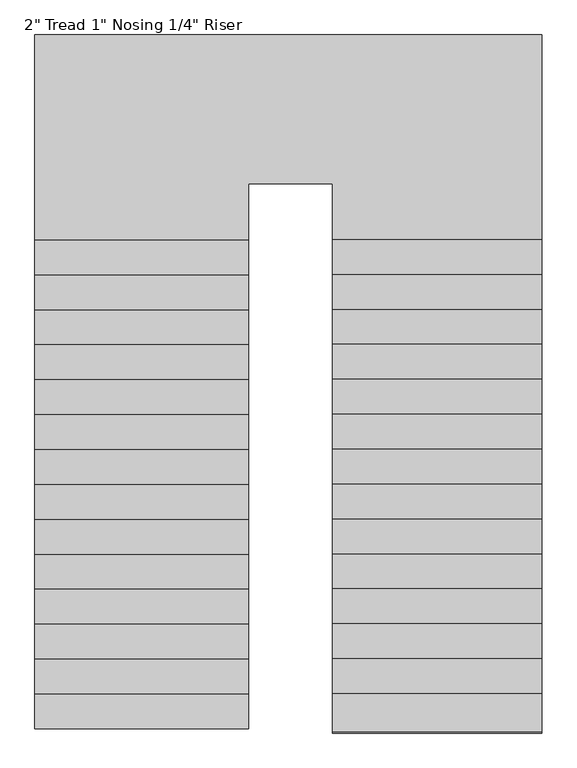
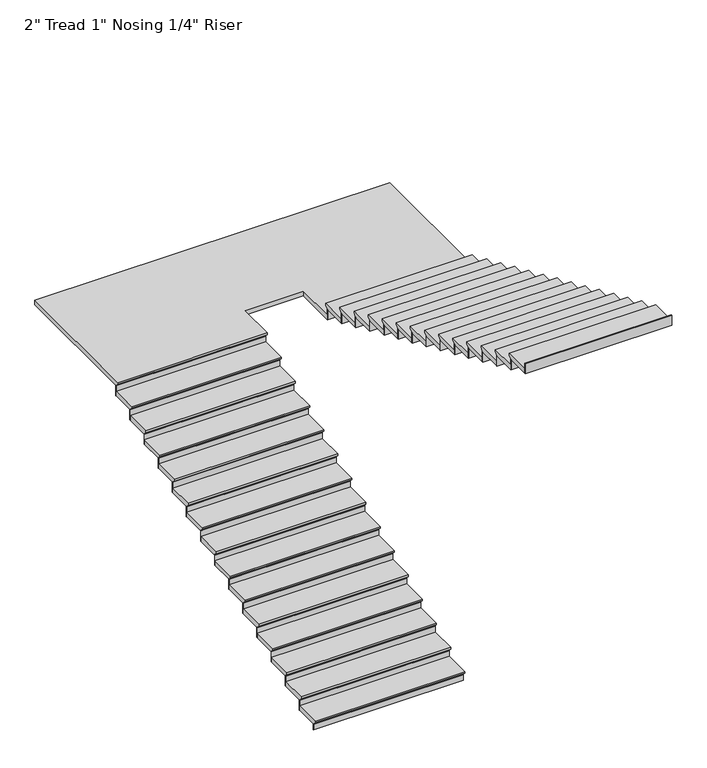
"""IFC4 building model written with IfcOpenShell, lengths in millimetres: stair flight geometry."""

from ifc_helpers import new_model, si_unit, origin, place, context, project, spatial, faceted_brep, source, transform, mapped, element, save


def stair_flight_303fa83b(model_context):
    return source(origin(), model_context, "Body", "Brep", [
        faceted_brep([(-5999.9290366, -6973.0610642, 11979.91), (-5999.9290366, -6973.0610642, 11998.96), (-7554.4415084, -6973.0610642, 11998.96), (-7554.4415084, -6973.0610642, 11979.91), (-5999.9290366, -6947.6610642, 11954.51), (-7554.4415084, -6947.6610642, 11954.51), (-5999.9290366, -6693.6610642, 11998.96), (-7554.4415084, -6693.6610642, 11998.96), (-7554.4415084, -6947.6610642, 11948.16), (-7554.4415084, -6693.6610642, 11948.16), (-5999.9290366, -6693.6610642, 11948.16), (-5999.9290366, -6947.6610642, 11948.16)], [[[0, 1, 2, 3]], [[4, 0, 3, 5]], [[2, 1, 6, 7]], [[8, 9, 10, 11]], [[2, 7, 9, 8, 5, 3]], [[8, 11, 4, 5]], [[6, 1, 0, 4, 11, 10]], [[7, 6, 10, 9]]]),
        faceted_brep([(-5999.9290366, -6947.6610642, 11948.16), (-5999.9290366, -6947.6610642, 11887.2), (-5999.9290366, -6941.3110642, 11887.2), (-5999.9290366, -6941.3110642, 11948.16), (-7554.4415084, -6947.6610642, 11948.16), (-7554.4415084, -6941.3110642, 11948.16), (-7554.4415084, -6941.3110642, 11887.2), (-7554.4415084, -6947.6610642, 11887.2)], [[[0, 1, 2, 3]], [[4, 5, 6, 7]], [[1, 0, 4, 7]], [[2, 1, 7, 6]], [[3, 2, 6, 5]], [[0, 3, 5, 4]]]),
        faceted_brep([(-5999.9290366, -6693.6610642, 12059.92), (-5999.9290366, -6693.6610642, 11948.16), (-5999.9290366, -6687.3110642, 11948.16), (-5999.9290366, -6687.3110642, 12059.92), (-7554.4415084, -6693.6610642, 12059.92), (-7554.4415084, -6687.3110642, 12059.92), (-7554.4415084, -6687.3110642, 11948.16), (-7554.4415084, -6693.6610642, 11948.16)], [[[0, 1, 2, 3]], [[4, 5, 6, 7]], [[1, 0, 4, 7]], [[2, 1, 7, 6]], [[3, 2, 6, 5]], [[0, 3, 5, 4]]]),
        faceted_brep([(-7554.4415084, -6719.0610642, 12110.72), (-5999.9290366, -6719.0610642, 12110.72), (-5999.9290366, -6439.6610642, 12110.72), (-7554.4415084, -6439.6610642, 12110.72), (-7554.4415084, -6693.6610642, 12059.92), (-7554.4415084, -6439.6610642, 12059.92), (-5999.9290366, -6439.6610642, 12059.92), (-5999.9290366, -6693.6610642, 12059.92), (-7554.4415084, -6693.6610642, 12066.27), (-7554.4415084, -6719.0610642, 12091.67), (-5999.9290366, -6693.6610642, 12066.27), (-5999.9290366, -6719.0610642, 12091.67)], [[[0, 1, 2, 3]], [[4, 5, 6, 7]], [[0, 3, 5, 4, 8, 9]], [[4, 7, 10, 8]], [[2, 1, 11, 10, 7, 6]], [[3, 2, 6, 5]], [[11, 1, 0, 9]], [[10, 11, 9, 8]]]),
        faceted_brep([(-5999.9290366, -6439.6610642, 12171.68), (-5999.9290366, -6439.6610642, 12059.92), (-5999.9290366, -6433.3110642, 12059.92), (-5999.9290366, -6433.3110642, 12171.68), (-7554.4415084, -6439.6610642, 12171.68), (-7554.4415084, -6433.3110642, 12171.68), (-7554.4415084, -6433.3110642, 12059.92), (-7554.4415084, -6439.6610642, 12059.92)], [[[0, 1, 2, 3]], [[4, 5, 6, 7]], [[1, 0, 4, 7]], [[2, 1, 7, 6]], [[3, 2, 6, 5]], [[0, 3, 5, 4]]]),
        faceted_brep([(-7554.4415084, -6465.0610642, 12222.48), (-5999.9290366, -6465.0610642, 12222.48), (-5999.9290366, -6185.6610642, 12222.48), (-7554.4415084, -6185.6610642, 12222.48), (-7554.4415084, -6439.6610642, 12171.68), (-7554.4415084, -6185.6610642, 12171.68), (-5999.9290366, -6185.6610642, 12171.68), (-5999.9290366, -6439.6610642, 12171.68), (-7554.4415084, -6439.6610642, 12178.03), (-7554.4415084, -6465.0610642, 12203.43), (-5999.9290366, -6439.6610642, 12178.03), (-5999.9290366, -6465.0610642, 12203.43)], [[[0, 1, 2, 3]], [[4, 5, 6, 7]], [[0, 3, 5, 4, 8, 9]], [[4, 7, 10, 8]], [[2, 1, 11, 10, 7, 6]], [[3, 2, 6, 5]], [[11, 1, 0, 9]], [[10, 11, 9, 8]]]),
        faceted_brep([(-5999.9290366, -6185.6610642, 12283.44), (-5999.9290366, -6185.6610642, 12171.68), (-5999.9290366, -6179.3110642, 12171.68), (-5999.9290366, -6179.3110642, 12283.44), (-7554.4415084, -6185.6610642, 12283.44), (-7554.4415084, -6179.3110642, 12283.44), (-7554.4415084, -6179.3110642, 12171.68), (-7554.4415084, -6185.6610642, 12171.68)], [[[0, 1, 2, 3]], [[4, 5, 6, 7]], [[1, 0, 4, 7]], [[2, 1, 7, 6]], [[3, 2, 6, 5]], [[0, 3, 5, 4]]]),
        faceted_brep([(-7554.4415084, -6211.0610642, 12334.24), (-5999.9290366, -6211.0610642, 12334.24), (-5999.9290366, -5931.6610642, 12334.24), (-7554.4415084, -5931.6610642, 12334.24), (-7554.4415084, -6185.6610642, 12283.44), (-7554.4415084, -5931.6610642, 12283.44), (-5999.9290366, -5931.6610642, 12283.44), (-5999.9290366, -6185.6610642, 12283.44), (-7554.4415084, -6185.6610642, 12289.79), (-7554.4415084, -6211.0610642, 12315.19), (-5999.9290366, -6185.6610642, 12289.79), (-5999.9290366, -6211.0610642, 12315.19)], [[[0, 1, 2, 3]], [[4, 5, 6, 7]], [[0, 3, 5, 4, 8, 9]], [[4, 7, 10, 8]], [[2, 1, 11, 10, 7, 6]], [[3, 2, 6, 5]], [[11, 1, 0, 9]], [[10, 11, 9, 8]]]),
        faceted_brep([(-5999.9290366, -5931.6610642, 12395.2), (-5999.9290366, -5931.6610642, 12283.44), (-5999.9290366, -5925.3110642, 12283.44), (-5999.9290366, -5925.3110642, 12395.2), (-7554.4415084, -5931.6610642, 12395.2), (-7554.4415084, -5925.3110642, 12395.2), (-7554.4415084, -5925.3110642, 12283.44), (-7554.4415084, -5931.6610642, 12283.44)], [[[0, 1, 2, 3]], [[4, 5, 6, 7]], [[1, 0, 4, 7]], [[2, 1, 7, 6]], [[3, 2, 6, 5]], [[0, 3, 5, 4]]]),
        faceted_brep([(-7554.4415084, -5957.0610642, 12446.0), (-5999.9290366, -5957.0610642, 12446.0), (-5999.9290366, -5677.6610642, 12446.0), (-7554.4415084, -5677.6610642, 12446.0), (-7554.4415084, -5931.6610642, 12395.2), (-7554.4415084, -5677.6610642, 12395.2), (-5999.9290366, -5677.6610642, 12395.2), (-5999.9290366, -5931.6610642, 12395.2), (-7554.4415084, -5931.6610642, 12401.55), (-7554.4415084, -5957.0610642, 12426.95), (-5999.9290366, -5931.6610642, 12401.55), (-5999.9290366, -5957.0610642, 12426.95)], [[[0, 1, 2, 3]], [[4, 5, 6, 7]], [[0, 3, 5, 4, 8, 9]], [[4, 7, 10, 8]], [[2, 1, 11, 10, 7, 6]], [[3, 2, 6, 5]], [[11, 1, 0, 9]], [[10, 11, 9, 8]]]),
        faceted_brep([(-5999.9290366, -5677.6610642, 12506.96), (-5999.9290366, -5677.6610642, 12395.2), (-5999.9290366, -5671.3110642, 12395.2), (-5999.9290366, -5671.3110642, 12506.96), (-7554.4415084, -5677.6610642, 12506.96), (-7554.4415084, -5671.3110642, 12506.96), (-7554.4415084, -5671.3110642, 12395.2), (-7554.4415084, -5677.6610642, 12395.2)], [[[0, 1, 2, 3]], [[4, 5, 6, 7]], [[1, 0, 4, 7]], [[2, 1, 7, 6]], [[3, 2, 6, 5]], [[0, 3, 5, 4]]]),
        faceted_brep([(-7554.4415084, -5703.0610642, 12557.76), (-5999.9290366, -5703.0610642, 12557.76), (-5999.9290366, -5423.6610642, 12557.76), (-7554.4415084, -5423.6610642, 12557.76), (-7554.4415084, -5677.6610642, 12506.96), (-7554.4415084, -5423.6610642, 12506.96), (-5999.9290366, -5423.6610642, 12506.96), (-5999.9290366, -5677.6610642, 12506.96), (-7554.4415084, -5677.6610642, 12513.31), (-7554.4415084, -5703.0610642, 12538.71), (-5999.9290366, -5677.6610642, 12513.31), (-5999.9290366, -5703.0610642, 12538.71)], [[[0, 1, 2, 3]], [[4, 5, 6, 7]], [[0, 3, 5, 4, 8, 9]], [[4, 7, 10, 8]], [[2, 1, 11, 10, 7, 6]], [[3, 2, 6, 5]], [[11, 1, 0, 9]], [[10, 11, 9, 8]]]),
        faceted_brep([(-5999.9290366, -5423.6610642, 12618.72), (-5999.9290366, -5423.6610642, 12506.96), (-5999.9290366, -5417.3110642, 12506.96), (-5999.9290366, -5417.3110642, 12618.72), (-7554.4415084, -5423.6610642, 12618.72), (-7554.4415084, -5417.3110642, 12618.72), (-7554.4415084, -5417.3110642, 12506.96), (-7554.4415084, -5423.6610642, 12506.96)], [[[0, 1, 2, 3]], [[4, 5, 6, 7]], [[1, 0, 4, 7]], [[2, 1, 7, 6]], [[3, 2, 6, 5]], [[0, 3, 5, 4]]]),
        faceted_brep([(-7554.4415084, -5449.0610642, 12669.52), (-5999.9290366, -5449.0610642, 12669.52), (-5999.9290366, -5169.6610642, 12669.52), (-7554.4415084, -5169.6610642, 12669.52), (-7554.4415084, -5423.6610642, 12618.72), (-7554.4415084, -5169.6610642, 12618.72), (-5999.9290366, -5169.6610642, 12618.72), (-5999.9290366, -5423.6610642, 12618.72), (-7554.4415084, -5423.6610642, 12625.07), (-7554.4415084, -5449.0610642, 12650.47), (-5999.9290366, -5423.6610642, 12625.07), (-5999.9290366, -5449.0610642, 12650.47)], [[[0, 1, 2, 3]], [[4, 5, 6, 7]], [[0, 3, 5, 4, 8, 9]], [[4, 7, 10, 8]], [[2, 1, 11, 10, 7, 6]], [[3, 2, 6, 5]], [[11, 1, 0, 9]], [[10, 11, 9, 8]]]),
        faceted_brep([(-5999.9290366, -5169.6610642, 12730.48), (-5999.9290366, -5169.6610642, 12618.72), (-5999.9290366, -5163.3110642, 12618.72), (-5999.9290366, -5163.3110642, 12730.48), (-7554.4415084, -5169.6610642, 12730.48), (-7554.4415084, -5163.3110642, 12730.48), (-7554.4415084, -5163.3110642, 12618.72), (-7554.4415084, -5169.6610642, 12618.72)], [[[0, 1, 2, 3]], [[4, 5, 6, 7]], [[1, 0, 4, 7]], [[2, 1, 7, 6]], [[3, 2, 6, 5]], [[0, 3, 5, 4]]]),
        faceted_brep([(-7554.4415084, -5195.0610642, 12781.28), (-5999.9290366, -5195.0610642, 12781.28), (-5999.9290366, -4915.6610642, 12781.28), (-7554.4415084, -4915.6610642, 12781.28), (-7554.4415084, -5169.6610642, 12730.48), (-7554.4415084, -4915.6610642, 12730.48), (-5999.9290366, -4915.6610642, 12730.48), (-5999.9290366, -5169.6610642, 12730.48), (-7554.4415084, -5169.6610642, 12736.83), (-7554.4415084, -5195.0610642, 12762.23), (-5999.9290366, -5169.6610642, 12736.83), (-5999.9290366, -5195.0610642, 12762.23)], [[[0, 1, 2, 3]], [[4, 5, 6, 7]], [[0, 3, 5, 4, 8, 9]], [[4, 7, 10, 8]], [[2, 1, 11, 10, 7, 6]], [[3, 2, 6, 5]], [[11, 1, 0, 9]], [[10, 11, 9, 8]]]),
        faceted_brep([(-5999.9290366, -4915.6610642, 12842.24), (-5999.9290366, -4915.6610642, 12730.48), (-5999.9290366, -4909.3110642, 12730.48), (-5999.9290366, -4909.3110642, 12842.24), (-7554.4415084, -4915.6610642, 12842.24), (-7554.4415084, -4909.3110642, 12842.24), (-7554.4415084, -4909.3110642, 12730.48), (-7554.4415084, -4915.6610642, 12730.48)], [[[0, 1, 2, 3]], [[4, 5, 6, 7]], [[1, 0, 4, 7]], [[2, 1, 7, 6]], [[3, 2, 6, 5]], [[0, 3, 5, 4]]]),
        faceted_brep([(-7554.4415084, -4941.0610642, 12893.04), (-5999.9290366, -4941.0610642, 12893.04), (-5999.9290366, -4661.6610642, 12893.04), (-7554.4415084, -4661.6610642, 12893.04), (-7554.4415084, -4915.6610642, 12842.24), (-7554.4415084, -4661.6610642, 12842.24), (-5999.9290366, -4661.6610642, 12842.24), (-5999.9290366, -4915.6610642, 12842.24), (-7554.4415084, -4915.6610642, 12848.59), (-7554.4415084, -4941.0610642, 12873.99), (-5999.9290366, -4915.6610642, 12848.59), (-5999.9290366, -4941.0610642, 12873.99)], [[[0, 1, 2, 3]], [[4, 5, 6, 7]], [[0, 3, 5, 4, 8, 9]], [[4, 7, 10, 8]], [[2, 1, 11, 10, 7, 6]], [[3, 2, 6, 5]], [[11, 1, 0, 9]], [[10, 11, 9, 8]]]),
        faceted_brep([(-5999.9290366, -4661.6610642, 12954.0), (-5999.9290366, -4661.6610642, 12842.24), (-5999.9290366, -4655.3110642, 12842.24), (-5999.9290366, -4655.3110642, 12954.0), (-7554.4415084, -4661.6610642, 12954.0), (-7554.4415084, -4655.3110642, 12954.0), (-7554.4415084, -4655.3110642, 12842.24), (-7554.4415084, -4661.6610642, 12842.24)], [[[0, 1, 2, 3]], [[4, 5, 6, 7]], [[1, 0, 4, 7]], [[2, 1, 7, 6]], [[3, 2, 6, 5]], [[0, 3, 5, 4]]]),
        faceted_brep([(-7554.4415084, -4687.0610642, 13004.8), (-5999.9290366, -4687.0610642, 13004.8), (-5999.9290366, -4407.6610642, 13004.8), (-7554.4415084, -4407.6610642, 13004.8), (-7554.4415084, -4661.6610642, 12954.0), (-7554.4415084, -4407.6610642, 12954.0), (-5999.9290366, -4407.6610642, 12954.0), (-5999.9290366, -4661.6610642, 12954.0), (-7554.4415084, -4661.6610642, 12960.35), (-7554.4415084, -4687.0610642, 12985.75), (-5999.9290366, -4661.6610642, 12960.35), (-5999.9290366, -4687.0610642, 12985.75)], [[[0, 1, 2, 3]], [[4, 5, 6, 7]], [[0, 3, 5, 4, 8, 9]], [[4, 7, 10, 8]], [[2, 1, 11, 10, 7, 6]], [[3, 2, 6, 5]], [[11, 1, 0, 9]], [[10, 11, 9, 8]]]),
        faceted_brep([(-5999.9290366, -4407.6610642, 13065.76), (-5999.9290366, -4407.6610642, 12954.0), (-5999.9290366, -4401.3110642, 12954.0), (-5999.9290366, -4401.3110642, 13065.76), (-7554.4415084, -4407.6610642, 13065.76), (-7554.4415084, -4401.3110642, 13065.76), (-7554.4415084, -4401.3110642, 12954.0), (-7554.4415084, -4407.6610642, 12954.0)], [[[0, 1, 2, 3]], [[4, 5, 6, 7]], [[1, 0, 4, 7]], [[2, 1, 7, 6]], [[3, 2, 6, 5]], [[0, 3, 5, 4]]]),
        faceted_brep([(-7554.4415084, -4433.0610642, 13116.56), (-5999.9290366, -4433.0610642, 13116.56), (-5999.9290366, -4153.6610642, 13116.56), (-7554.4415084, -4153.6610642, 13116.56), (-7554.4415084, -4407.6610642, 13065.76), (-7554.4415084, -4153.6610642, 13065.76), (-5999.9290366, -4153.6610642, 13065.76), (-5999.9290366, -4407.6610642, 13065.76), (-7554.4415084, -4407.6610642, 13072.11), (-7554.4415084, -4433.0610642, 13097.51), (-5999.9290366, -4407.6610642, 13072.11), (-5999.9290366, -4433.0610642, 13097.51)], [[[0, 1, 2, 3]], [[4, 5, 6, 7]], [[0, 3, 5, 4, 8, 9]], [[4, 7, 10, 8]], [[2, 1, 11, 10, 7, 6]], [[3, 2, 6, 5]], [[11, 1, 0, 9]], [[10, 11, 9, 8]]]),
        faceted_brep([(-5999.9290366, -4153.6610642, 13177.52), (-5999.9290366, -4153.6610642, 13065.76), (-5999.9290366, -4147.3110642, 13065.76), (-5999.9290366, -4147.3110642, 13177.52), (-7554.4415084, -4153.6610642, 13177.52), (-7554.4415084, -4147.3110642, 13177.52), (-7554.4415084, -4147.3110642, 13065.76), (-7554.4415084, -4153.6610642, 13065.76)], [[[0, 1, 2, 3]], [[4, 5, 6, 7]], [[1, 0, 4, 7]], [[2, 1, 7, 6]], [[3, 2, 6, 5]], [[0, 3, 5, 4]]]),
        faceted_brep([(-7554.4415084, -4179.0610642, 13228.32), (-5999.9290366, -4179.0610642, 13228.32), (-5999.9290366, -3899.6610642, 13228.32), (-7554.4415084, -3899.6610642, 13228.32), (-7554.4415084, -4153.6610642, 13177.52), (-7554.4415084, -3899.6610642, 13177.52), (-5999.9290366, -3899.6610642, 13177.52), (-5999.9290366, -4153.6610642, 13177.52), (-7554.4415084, -4153.6610642, 13183.87), (-7554.4415084, -4179.0610642, 13209.27), (-5999.9290366, -4153.6610642, 13183.87), (-5999.9290366, -4179.0610642, 13209.27)], [[[0, 1, 2, 3]], [[4, 5, 6, 7]], [[0, 3, 5, 4, 8, 9]], [[4, 7, 10, 8]], [[2, 1, 11, 10, 7, 6]], [[3, 2, 6, 5]], [[11, 1, 0, 9]], [[10, 11, 9, 8]]]),
        faceted_brep([(-5999.9290366, -3899.6610642, 13289.28), (-5999.9290366, -3899.6610642, 13177.52), (-5999.9290366, -3893.3110642, 13177.52), (-5999.9290366, -3893.3110642, 13289.28), (-7554.4415084, -3899.6610642, 13289.28), (-7554.4415084, -3893.3110642, 13289.28), (-7554.4415084, -3893.3110642, 13177.52), (-7554.4415084, -3899.6610642, 13177.52)], [[[0, 1, 2, 3]], [[4, 5, 6, 7]], [[1, 0, 4, 7]], [[2, 1, 7, 6]], [[3, 2, 6, 5]], [[0, 3, 5, 4]]]),
        faceted_brep([(-7554.4415084, -3925.0610642, 13340.08), (-5999.9290366, -3925.0610642, 13340.08), (-5999.9290366, -3645.6610642, 13340.08), (-7554.4415084, -3645.6610642, 13340.08), (-7554.4415084, -3899.6610642, 13289.28), (-7554.4415084, -3645.6610642, 13289.28), (-5999.9290366, -3645.6610642, 13289.28), (-5999.9290366, -3899.6610642, 13289.28), (-7554.4415084, -3899.6610642, 13295.63), (-7554.4415084, -3925.0610642, 13321.03), (-5999.9290366, -3899.6610642, 13295.63), (-5999.9290366, -3925.0610642, 13321.03)], [[[0, 1, 2, 3]], [[4, 5, 6, 7]], [[0, 3, 5, 4, 8, 9]], [[4, 7, 10, 8]], [[2, 1, 11, 10, 7, 6]], [[3, 2, 6, 5]], [[11, 1, 0, 9]], [[10, 11, 9, 8]]]),
        faceted_brep([(-5999.9290366, -3645.6610642, 13401.04), (-5999.9290366, -3645.6610642, 13289.28), (-5999.9290366, -3639.3110642, 13289.28), (-5999.9290366, -3639.3110642, 13401.04), (-7554.4415084, -3645.6610642, 13401.04), (-7554.4415084, -3639.3110642, 13401.04), (-7554.4415084, -3639.3110642, 13289.28), (-7554.4415084, -3645.6610642, 13289.28)], [[[0, 1, 2, 3]], [[4, 5, 6, 7]], [[1, 0, 4, 7]], [[2, 1, 7, 6]], [[3, 2, 6, 5]], [[0, 3, 5, 4]]]),
        faceted_brep([(-7554.4415084, -3671.0610642, 13451.84), (-5999.9290366, -3671.0610642, 13451.84), (-5999.9290366, -3391.6610642, 13451.84), (-7554.4415084, -3391.6610642, 13451.84), (-7554.4415084, -3645.6610642, 13401.04), (-7554.4415084, -3391.6610642, 13401.04), (-5999.9290366, -3391.6610642, 13401.04), (-5999.9290366, -3645.6610642, 13401.04), (-7554.4415084, -3645.6610642, 13407.39), (-7554.4415084, -3671.0610642, 13432.79), (-5999.9290366, -3645.6610642, 13407.39), (-5999.9290366, -3671.0610642, 13432.79)], [[[0, 1, 2, 3]], [[4, 5, 6, 7]], [[0, 3, 5, 4, 8, 9]], [[4, 7, 10, 8]], [[2, 1, 11, 10, 7, 6]], [[3, 2, 6, 5]], [[11, 1, 0, 9]], [[10, 11, 9, 8]]]),
        faceted_brep([(-5999.9290366, -3391.6610642, 13512.8), (-5999.9290366, -3391.6610642, 13401.04), (-5999.9290366, -3385.3110642, 13401.04), (-5999.9290366, -3385.3110642, 13512.8), (-7554.4415084, -3391.6610642, 13512.8), (-7554.4415084, -3385.3110642, 13512.8), (-7554.4415084, -3385.3110642, 13401.04), (-7554.4415084, -3391.6610642, 13401.04)], [[[0, 1, 2, 3]], [[4, 5, 6, 7]], [[1, 0, 4, 7]], [[2, 1, 7, 6]], [[3, 2, 6, 5]], [[0, 3, 5, 4]]]),
        faceted_brep([(-3866.3290366, -3442.4610642, 13563.6), (-3866.3290366, -1928.4217109, 13563.6), (-7554.4415084, -1928.4217109, 13563.6), (-7554.4415084, -3417.0610642, 13563.6), (-5999.9290366, -3417.0610642, 13563.6), (-5999.9290366, -3010.6610642, 13563.6), (-5390.3290366, -3010.6610642, 13563.6), (-5390.3290366, -3442.4610642, 13563.6), (-3866.3290366, -1928.4217109, 13512.8), (-3866.3290366, -3442.4610642, 13512.8), (-5390.3290366, -3442.4610642, 13512.8), (-5390.3290366, -3010.6610642, 13512.8), (-5999.9290366, -3010.6610642, 13512.8), (-5999.9290366, -3391.6610642, 13512.8), (-7554.4415084, -3391.6610642, 13512.8), (-7554.4415084, -1928.4217109, 13512.8), (-7554.4415084, -3391.6610642, 13519.15), (-7554.4415084, -3417.0610642, 13544.55), (-5999.9290366, -3391.6610642, 13519.15), (-5999.9290366, -3417.0610642, 13544.55)], [[[0, 1, 2, 3, 4, 5, 6, 7]], [[8, 9, 10, 11, 12, 13, 14, 15]], [[1, 0, 9, 8]], [[2, 1, 8, 15]], [[3, 2, 15, 14, 16, 17]], [[14, 13, 18, 16]], [[5, 4, 19, 18, 13, 12]], [[6, 5, 12, 11]], [[7, 6, 11, 10]], [[0, 7, 10, 9]], [[19, 4, 3, 17]], [[18, 19, 17, 16]]]),
        faceted_brep([(-5390.3290366, -3442.4610642, 13624.56), (-5390.3290366, -3442.4610642, 13512.8), (-5390.3290366, -3448.8110642, 13512.8), (-5390.3290366, -3448.8110642, 13624.56), (-3866.3290366, -3442.4610642, 13624.56), (-3866.3290366, -3448.8110642, 13624.56), (-3866.3290366, -3448.8110642, 13512.8), (-3866.3290366, -3442.4610642, 13512.8)], [[[0, 1, 2, 3]], [[4, 5, 6, 7]], [[1, 0, 4, 7]], [[2, 1, 7, 6]], [[3, 2, 6, 5]], [[0, 3, 5, 4]]]),
        faceted_brep([(-3866.3290366, -3417.0610642, 13675.36), (-5390.3290366, -3417.0610642, 13675.36), (-5390.3290366, -3696.4610642, 13675.36), (-3866.3290366, -3696.4610642, 13675.36), (-3866.3290366, -3442.4610642, 13624.56), (-3866.3290366, -3696.4610642, 13624.56), (-5390.3290366, -3696.4610642, 13624.56), (-5390.3290366, -3442.4610642, 13624.56), (-3866.3290366, -3442.4610642, 13630.91), (-3866.3290366, -3417.0610642, 13656.31), (-5390.3290366, -3442.4610642, 13630.91), (-5390.3290366, -3417.0610642, 13656.31)], [[[0, 1, 2, 3]], [[4, 5, 6, 7]], [[0, 3, 5, 4, 8, 9]], [[4, 7, 10, 8]], [[2, 1, 11, 10, 7, 6]], [[3, 2, 6, 5]], [[11, 1, 0, 9]], [[10, 11, 9, 8]]]),
        faceted_brep([(-5390.3290366, -3696.4610642, 13736.32), (-5390.3290366, -3696.4610642, 13624.56), (-5390.3290366, -3702.8110642, 13624.56), (-5390.3290366, -3702.8110642, 13736.32), (-3866.3290366, -3696.4610642, 13736.32), (-3866.3290366, -3702.8110642, 13736.32), (-3866.3290366, -3702.8110642, 13624.56), (-3866.3290366, -3696.4610642, 13624.56)], [[[0, 1, 2, 3]], [[4, 5, 6, 7]], [[1, 0, 4, 7]], [[2, 1, 7, 6]], [[3, 2, 6, 5]], [[0, 3, 5, 4]]]),
        faceted_brep([(-3866.3290366, -3671.0610642, 13787.12), (-5390.3290366, -3671.0610642, 13787.12), (-5390.3290366, -3950.4610642, 13787.12), (-3866.3290366, -3950.4610642, 13787.12), (-3866.3290366, -3696.4610642, 13736.32), (-3866.3290366, -3950.4610642, 13736.32), (-5390.3290366, -3950.4610642, 13736.32), (-5390.3290366, -3696.4610642, 13736.32), (-3866.3290366, -3696.4610642, 13742.67), (-3866.3290366, -3671.0610642, 13768.07), (-5390.3290366, -3696.4610642, 13742.67), (-5390.3290366, -3671.0610642, 13768.07)], [[[0, 1, 2, 3]], [[4, 5, 6, 7]], [[0, 3, 5, 4, 8, 9]], [[4, 7, 10, 8]], [[2, 1, 11, 10, 7, 6]], [[3, 2, 6, 5]], [[11, 1, 0, 9]], [[10, 11, 9, 8]]]),
        faceted_brep([(-5390.3290366, -3950.4610642, 13848.08), (-5390.3290366, -3950.4610642, 13736.32), (-5390.3290366, -3956.8110642, 13736.32), (-5390.3290366, -3956.8110642, 13848.08), (-3866.3290366, -3950.4610642, 13848.08), (-3866.3290366, -3956.8110642, 13848.08), (-3866.3290366, -3956.8110642, 13736.32), (-3866.3290366, -3950.4610642, 13736.32)], [[[0, 1, 2, 3]], [[4, 5, 6, 7]], [[1, 0, 4, 7]], [[2, 1, 7, 6]], [[3, 2, 6, 5]], [[0, 3, 5, 4]]]),
        faceted_brep([(-3866.3290366, -3925.0610642, 13898.88), (-5390.3290366, -3925.0610642, 13898.88), (-5390.3290366, -4204.4610642, 13898.88), (-3866.3290366, -4204.4610642, 13898.88), (-3866.3290366, -3950.4610642, 13848.08), (-3866.3290366, -4204.4610642, 13848.08), (-5390.3290366, -4204.4610642, 13848.08), (-5390.3290366, -3950.4610642, 13848.08), (-3866.3290366, -3950.4610642, 13854.43), (-3866.3290366, -3925.0610642, 13879.83), (-5390.3290366, -3950.4610642, 13854.43), (-5390.3290366, -3925.0610642, 13879.83)], [[[0, 1, 2, 3]], [[4, 5, 6, 7]], [[0, 3, 5, 4, 8, 9]], [[4, 7, 10, 8]], [[2, 1, 11, 10, 7, 6]], [[3, 2, 6, 5]], [[11, 1, 0, 9]], [[10, 11, 9, 8]]]),
        faceted_brep([(-5390.3290366, -4204.4610642, 13959.84), (-5390.3290366, -4204.4610642, 13848.08), (-5390.3290366, -4210.8110642, 13848.08), (-5390.3290366, -4210.8110642, 13959.84), (-3866.3290366, -4204.4610642, 13959.84), (-3866.3290366, -4210.8110642, 13959.84), (-3866.3290366, -4210.8110642, 13848.08), (-3866.3290366, -4204.4610642, 13848.08)], [[[0, 1, 2, 3]], [[4, 5, 6, 7]], [[1, 0, 4, 7]], [[2, 1, 7, 6]], [[3, 2, 6, 5]], [[0, 3, 5, 4]]]),
        faceted_brep([(-3866.3290366, -4179.0610642, 14010.64), (-5390.3290366, -4179.0610642, 14010.64), (-5390.3290366, -4458.4610642, 14010.64), (-3866.3290366, -4458.4610642, 14010.64), (-3866.3290366, -4204.4610642, 13959.84), (-3866.3290366, -4458.4610642, 13959.84), (-5390.3290366, -4458.4610642, 13959.84), (-5390.3290366, -4204.4610642, 13959.84), (-3866.3290366, -4204.4610642, 13966.19), (-3866.3290366, -4179.0610642, 13991.59), (-5390.3290366, -4204.4610642, 13966.19), (-5390.3290366, -4179.0610642, 13991.59)], [[[0, 1, 2, 3]], [[4, 5, 6, 7]], [[0, 3, 5, 4, 8, 9]], [[4, 7, 10, 8]], [[2, 1, 11, 10, 7, 6]], [[3, 2, 6, 5]], [[11, 1, 0, 9]], [[10, 11, 9, 8]]]),
        faceted_brep([(-5390.3290366, -4458.4610642, 14071.6), (-5390.3290366, -4458.4610642, 13959.84), (-5390.3290366, -4464.8110642, 13959.84), (-5390.3290366, -4464.8110642, 14071.6), (-3866.3290366, -4458.4610642, 14071.6), (-3866.3290366, -4464.8110642, 14071.6), (-3866.3290366, -4464.8110642, 13959.84), (-3866.3290366, -4458.4610642, 13959.84)], [[[0, 1, 2, 3]], [[4, 5, 6, 7]], [[1, 0, 4, 7]], [[2, 1, 7, 6]], [[3, 2, 6, 5]], [[0, 3, 5, 4]]]),
        faceted_brep([(-3866.3290366, -4433.0610642, 14122.4), (-5390.3290366, -4433.0610642, 14122.4), (-5390.3290366, -4712.4610642, 14122.4), (-3866.3290366, -4712.4610642, 14122.4), (-3866.3290366, -4458.4610642, 14071.6), (-3866.3290366, -4712.4610642, 14071.6), (-5390.3290366, -4712.4610642, 14071.6), (-5390.3290366, -4458.4610642, 14071.6), (-3866.3290366, -4458.4610642, 14077.95), (-3866.3290366, -4433.0610642, 14103.35), (-5390.3290366, -4458.4610642, 14077.95), (-5390.3290366, -4433.0610642, 14103.35)], [[[0, 1, 2, 3]], [[4, 5, 6, 7]], [[0, 3, 5, 4, 8, 9]], [[4, 7, 10, 8]], [[2, 1, 11, 10, 7, 6]], [[3, 2, 6, 5]], [[11, 1, 0, 9]], [[10, 11, 9, 8]]]),
        faceted_brep([(-5390.3290366, -4712.4610642, 14183.36), (-5390.3290366, -4712.4610642, 14071.6), (-5390.3290366, -4718.8110642, 14071.6), (-5390.3290366, -4718.8110642, 14183.36), (-3866.3290366, -4712.4610642, 14183.36), (-3866.3290366, -4718.8110642, 14183.36), (-3866.3290366, -4718.8110642, 14071.6), (-3866.3290366, -4712.4610642, 14071.6)], [[[0, 1, 2, 3]], [[4, 5, 6, 7]], [[1, 0, 4, 7]], [[2, 1, 7, 6]], [[3, 2, 6, 5]], [[0, 3, 5, 4]]]),
        faceted_brep([(-3866.3290366, -4687.0610642, 14234.16), (-5390.3290366, -4687.0610642, 14234.16), (-5390.3290366, -4966.4610642, 14234.16), (-3866.3290366, -4966.4610642, 14234.16), (-3866.3290366, -4712.4610642, 14183.36), (-3866.3290366, -4966.4610642, 14183.36), (-5390.3290366, -4966.4610642, 14183.36), (-5390.3290366, -4712.4610642, 14183.36), (-3866.3290366, -4712.4610642, 14189.71), (-3866.3290366, -4687.0610642, 14215.11), (-5390.3290366, -4712.4610642, 14189.71), (-5390.3290366, -4687.0610642, 14215.11)], [[[0, 1, 2, 3]], [[4, 5, 6, 7]], [[0, 3, 5, 4, 8, 9]], [[4, 7, 10, 8]], [[2, 1, 11, 10, 7, 6]], [[3, 2, 6, 5]], [[11, 1, 0, 9]], [[10, 11, 9, 8]]]),
        faceted_brep([(-5390.3290366, -4966.4610642, 14295.12), (-5390.3290366, -4966.4610642, 14183.36), (-5390.3290366, -4972.8110642, 14183.36), (-5390.3290366, -4972.8110642, 14295.12), (-3866.3290366, -4966.4610642, 14295.12), (-3866.3290366, -4972.8110642, 14295.12), (-3866.3290366, -4972.8110642, 14183.36), (-3866.3290366, -4966.4610642, 14183.36)], [[[0, 1, 2, 3]], [[4, 5, 6, 7]], [[1, 0, 4, 7]], [[2, 1, 7, 6]], [[3, 2, 6, 5]], [[0, 3, 5, 4]]]),
        faceted_brep([(-3866.3290366, -4941.0610642, 14345.92), (-5390.3290366, -4941.0610642, 14345.92), (-5390.3290366, -5220.4610642, 14345.92), (-3866.3290366, -5220.4610642, 14345.92), (-3866.3290366, -4966.4610642, 14295.12), (-3866.3290366, -5220.4610642, 14295.12), (-5390.3290366, -5220.4610642, 14295.12), (-5390.3290366, -4966.4610642, 14295.12), (-3866.3290366, -4966.4610642, 14301.47), (-3866.3290366, -4941.0610642, 14326.87), (-5390.3290366, -4966.4610642, 14301.47), (-5390.3290366, -4941.0610642, 14326.87)], [[[0, 1, 2, 3]], [[4, 5, 6, 7]], [[0, 3, 5, 4, 8, 9]], [[4, 7, 10, 8]], [[2, 1, 11, 10, 7, 6]], [[3, 2, 6, 5]], [[11, 1, 0, 9]], [[10, 11, 9, 8]]]),
        faceted_brep([(-5390.3290366, -5220.4610642, 14406.88), (-5390.3290366, -5220.4610642, 14295.12), (-5390.3290366, -5226.8110642, 14295.12), (-5390.3290366, -5226.8110642, 14406.88), (-3866.3290366, -5220.4610642, 14406.88), (-3866.3290366, -5226.8110642, 14406.88), (-3866.3290366, -5226.8110642, 14295.12), (-3866.3290366, -5220.4610642, 14295.12)], [[[0, 1, 2, 3]], [[4, 5, 6, 7]], [[1, 0, 4, 7]], [[2, 1, 7, 6]], [[3, 2, 6, 5]], [[0, 3, 5, 4]]]),
        faceted_brep([(-3866.3290366, -5195.0610642, 14457.68), (-5390.3290366, -5195.0610642, 14457.68), (-5390.3290366, -5474.4610642, 14457.68), (-3866.3290366, -5474.4610642, 14457.68), (-3866.3290366, -5220.4610642, 14406.88), (-3866.3290366, -5474.4610642, 14406.88), (-5390.3290366, -5474.4610642, 14406.88), (-5390.3290366, -5220.4610642, 14406.88), (-3866.3290366, -5220.4610642, 14413.23), (-3866.3290366, -5195.0610642, 14438.63), (-5390.3290366, -5220.4610642, 14413.23), (-5390.3290366, -5195.0610642, 14438.63)], [[[0, 1, 2, 3]], [[4, 5, 6, 7]], [[0, 3, 5, 4, 8, 9]], [[4, 7, 10, 8]], [[2, 1, 11, 10, 7, 6]], [[3, 2, 6, 5]], [[11, 1, 0, 9]], [[10, 11, 9, 8]]]),
        faceted_brep([(-5390.3290366, -5474.4610642, 14518.64), (-5390.3290366, -5474.4610642, 14406.88), (-5390.3290366, -5480.8110642, 14406.88), (-5390.3290366, -5480.8110642, 14518.64), (-3866.3290366, -5474.4610642, 14518.64), (-3866.3290366, -5480.8110642, 14518.64), (-3866.3290366, -5480.8110642, 14406.88), (-3866.3290366, -5474.4610642, 14406.88)], [[[0, 1, 2, 3]], [[4, 5, 6, 7]], [[1, 0, 4, 7]], [[2, 1, 7, 6]], [[3, 2, 6, 5]], [[0, 3, 5, 4]]]),
        faceted_brep([(-3866.3290366, -5449.0610642, 14569.44), (-5390.3290366, -5449.0610642, 14569.44), (-5390.3290366, -5728.4610642, 14569.44), (-3866.3290366, -5728.4610642, 14569.44), (-3866.3290366, -5474.4610642, 14518.64), (-3866.3290366, -5728.4610642, 14518.64), (-5390.3290366, -5728.4610642, 14518.64), (-5390.3290366, -5474.4610642, 14518.64), (-3866.3290366, -5474.4610642, 14524.99), (-3866.3290366, -5449.0610642, 14550.39), (-5390.3290366, -5474.4610642, 14524.99), (-5390.3290366, -5449.0610642, 14550.39)], [[[0, 1, 2, 3]], [[4, 5, 6, 7]], [[0, 3, 5, 4, 8, 9]], [[4, 7, 10, 8]], [[2, 1, 11, 10, 7, 6]], [[3, 2, 6, 5]], [[11, 1, 0, 9]], [[10, 11, 9, 8]]]),
        faceted_brep([(-5390.3290366, -5728.4610642, 14630.4), (-5390.3290366, -5728.4610642, 14518.64), (-5390.3290366, -5734.8110642, 14518.64), (-5390.3290366, -5734.8110642, 14630.4), (-3866.3290366, -5728.4610642, 14630.4), (-3866.3290366, -5734.8110642, 14630.4), (-3866.3290366, -5734.8110642, 14518.64), (-3866.3290366, -5728.4610642, 14518.64)], [[[0, 1, 2, 3]], [[4, 5, 6, 7]], [[1, 0, 4, 7]], [[2, 1, 7, 6]], [[3, 2, 6, 5]], [[0, 3, 5, 4]]]),
        faceted_brep([(-3866.3290366, -5703.0610642, 14681.2), (-5390.3290366, -5703.0610642, 14681.2), (-5390.3290366, -5982.4610642, 14681.2), (-3866.3290366, -5982.4610642, 14681.2), (-3866.3290366, -5728.4610642, 14630.4), (-3866.3290366, -5982.4610642, 14630.4), (-5390.3290366, -5982.4610642, 14630.4), (-5390.3290366, -5728.4610642, 14630.4), (-3866.3290366, -5728.4610642, 14636.75), (-3866.3290366, -5703.0610642, 14662.15), (-5390.3290366, -5728.4610642, 14636.75), (-5390.3290366, -5703.0610642, 14662.15)], [[[0, 1, 2, 3]], [[4, 5, 6, 7]], [[0, 3, 5, 4, 8, 9]], [[4, 7, 10, 8]], [[2, 1, 11, 10, 7, 6]], [[3, 2, 6, 5]], [[11, 1, 0, 9]], [[10, 11, 9, 8]]]),
        faceted_brep([(-5390.3290366, -5982.4610642, 14742.16), (-5390.3290366, -5982.4610642, 14630.4), (-5390.3290366, -5988.8110642, 14630.4), (-5390.3290366, -5988.8110642, 14742.16), (-3866.3290366, -5982.4610642, 14742.16), (-3866.3290366, -5988.8110642, 14742.16), (-3866.3290366, -5988.8110642, 14630.4), (-3866.3290366, -5982.4610642, 14630.4)], [[[0, 1, 2, 3]], [[4, 5, 6, 7]], [[1, 0, 4, 7]], [[2, 1, 7, 6]], [[3, 2, 6, 5]], [[0, 3, 5, 4]]]),
        faceted_brep([(-3866.3290366, -5957.0610642, 14792.96), (-5390.3290366, -5957.0610642, 14792.96), (-5390.3290366, -6236.4610642, 14792.96), (-3866.3290366, -6236.4610642, 14792.96), (-3866.3290366, -5982.4610642, 14742.16), (-3866.3290366, -6236.4610642, 14742.16), (-5390.3290366, -6236.4610642, 14742.16), (-5390.3290366, -5982.4610642, 14742.16), (-3866.3290366, -5982.4610642, 14748.51), (-3866.3290366, -5957.0610642, 14773.91), (-5390.3290366, -5982.4610642, 14748.51), (-5390.3290366, -5957.0610642, 14773.91)], [[[0, 1, 2, 3]], [[4, 5, 6, 7]], [[0, 3, 5, 4, 8, 9]], [[4, 7, 10, 8]], [[2, 1, 11, 10, 7, 6]], [[3, 2, 6, 5]], [[11, 1, 0, 9]], [[10, 11, 9, 8]]]),
        faceted_brep([(-5390.3290366, -6236.4610642, 14853.92), (-5390.3290366, -6236.4610642, 14742.16), (-5390.3290366, -6242.8110642, 14742.16), (-5390.3290366, -6242.8110642, 14853.92), (-3866.3290366, -6236.4610642, 14853.92), (-3866.3290366, -6242.8110642, 14853.92), (-3866.3290366, -6242.8110642, 14742.16), (-3866.3290366, -6236.4610642, 14742.16)], [[[0, 1, 2, 3]], [[4, 5, 6, 7]], [[1, 0, 4, 7]], [[2, 1, 7, 6]], [[3, 2, 6, 5]], [[0, 3, 5, 4]]]),
        faceted_brep([(-3866.3290366, -6211.0610642, 14904.72), (-5390.3290366, -6211.0610642, 14904.72), (-5390.3290366, -6490.4610642, 14904.72), (-3866.3290366, -6490.4610642, 14904.72), (-3866.3290366, -6236.4610642, 14853.92), (-3866.3290366, -6490.4610642, 14853.92), (-5390.3290366, -6490.4610642, 14853.92), (-5390.3290366, -6236.4610642, 14853.92), (-3866.3290366, -6236.4610642, 14860.27), (-3866.3290366, -6211.0610642, 14885.67), (-5390.3290366, -6236.4610642, 14860.27), (-5390.3290366, -6211.0610642, 14885.67)], [[[0, 1, 2, 3]], [[4, 5, 6, 7]], [[0, 3, 5, 4, 8, 9]], [[4, 7, 10, 8]], [[2, 1, 11, 10, 7, 6]], [[3, 2, 6, 5]], [[11, 1, 0, 9]], [[10, 11, 9, 8]]]),
        faceted_brep([(-5390.3290366, -6490.4610642, 14965.68), (-5390.3290366, -6490.4610642, 14853.92), (-5390.3290366, -6496.8110642, 14853.92), (-5390.3290366, -6496.8110642, 14965.68), (-3866.3290366, -6490.4610642, 14965.68), (-3866.3290366, -6496.8110642, 14965.68), (-3866.3290366, -6496.8110642, 14853.92), (-3866.3290366, -6490.4610642, 14853.92)], [[[0, 1, 2, 3]], [[4, 5, 6, 7]], [[1, 0, 4, 7]], [[2, 1, 7, 6]], [[3, 2, 6, 5]], [[0, 3, 5, 4]]]),
        faceted_brep([(-3866.3290366, -6465.0610642, 15016.48), (-5390.3290366, -6465.0610642, 15016.48), (-5390.3290366, -6744.4610642, 15016.48), (-3866.3290366, -6744.4610642, 15016.48), (-3866.3290366, -6490.4610642, 14965.68), (-3866.3290366, -6744.4610642, 14965.68), (-5390.3290366, -6744.4610642, 14965.68), (-5390.3290366, -6490.4610642, 14965.68), (-3866.3290366, -6490.4610642, 14972.03), (-3866.3290366, -6465.0610642, 14997.43), (-5390.3290366, -6490.4610642, 14972.03), (-5390.3290366, -6465.0610642, 14997.43)], [[[0, 1, 2, 3]], [[4, 5, 6, 7]], [[0, 3, 5, 4, 8, 9]], [[4, 7, 10, 8]], [[2, 1, 11, 10, 7, 6]], [[3, 2, 6, 5]], [[11, 1, 0, 9]], [[10, 11, 9, 8]]]),
        faceted_brep([(-5390.3290366, -6744.4610642, 15077.44), (-5390.3290366, -6744.4610642, 14965.68), (-5390.3290366, -6750.8110642, 14965.68), (-5390.3290366, -6750.8110642, 15077.44), (-3866.3290366, -6744.4610642, 15077.44), (-3866.3290366, -6750.8110642, 15077.44), (-3866.3290366, -6750.8110642, 14965.68), (-3866.3290366, -6744.4610642, 14965.68)], [[[0, 1, 2, 3]], [[4, 5, 6, 7]], [[1, 0, 4, 7]], [[2, 1, 7, 6]], [[3, 2, 6, 5]], [[0, 3, 5, 4]]]),
        faceted_brep([(-5390.3290366, -6998.4610642, 15189.2), (-5390.3290366, -6998.4610642, 15077.44), (-5390.3290366, -7004.8110642, 15077.44), (-5390.3290366, -7004.8110642, 15189.2), (-3866.3290366, -6998.4610642, 15189.2), (-3866.3290366, -7004.8110642, 15189.2), (-3866.3290366, -7004.8110642, 15077.44), (-3866.3290366, -6998.4610642, 15077.44)], [[[0, 1, 2, 3]], [[4, 5, 6, 7]], [[1, 0, 4, 7]], [[2, 1, 7, 6]], [[3, 2, 6, 5]], [[0, 3, 5, 4]]]),
        faceted_brep([(-3866.3290366, -6719.0610642, 15128.24), (-5390.3290366, -6719.0610642, 15128.24), (-5390.3290366, -6998.4610642, 15128.24), (-3866.3290366, -6998.4610642, 15128.24), (-3866.3290366, -6744.4610642, 15077.44), (-3866.3290366, -6998.4610642, 15077.44), (-5390.3290366, -6998.4610642, 15077.44), (-5390.3290366, -6744.4610642, 15077.44), (-3866.3290366, -6744.4610642, 15083.79), (-3866.3290366, -6719.0610642, 15109.19), (-5390.3290366, -6744.4610642, 15083.79), (-5390.3290366, -6719.0610642, 15109.19)], [[[0, 1, 2, 3]], [[4, 5, 6, 7]], [[0, 3, 5, 4, 8, 9]], [[4, 7, 10, 8]], [[2, 1, 11, 10, 7, 6]], [[3, 2, 6, 5]], [[11, 1, 0, 9]], [[10, 11, 9, 8]]]),
    ])


if __name__ == "__main__":
    model = new_model("IFC4")
    model_context = context("Model", 3, world=origin())
    ifc_project = project(units=[si_unit("LENGTHUNIT", "METRE", prefix="MILLI")], contexts=[model_context])
    site = spatial("IfcSite", under=ifc_project)
    building = spatial("IfcBuilding", under=site)
    placement = place(None, origin())
    stair_flight_shape = stair_flight_303fa83b(model_context)
    element("IfcStairFlight", 1, ObjectType="2\" Tread 1\" Nosing 1/4\" Riser", at=placement, inside=building, context=model_context, shape_type="MappedRepresentation", body=[
        mapped(stair_flight_shape, transform((0.0, 0.0, 0.0), x_axis=(1.0, 0.0, 0.0), y_axis=(0.0, 1.0, 0.0), z_axis=(0.0, 0.0, 1.0))),
    ])
    save(model, "model.ifc")
